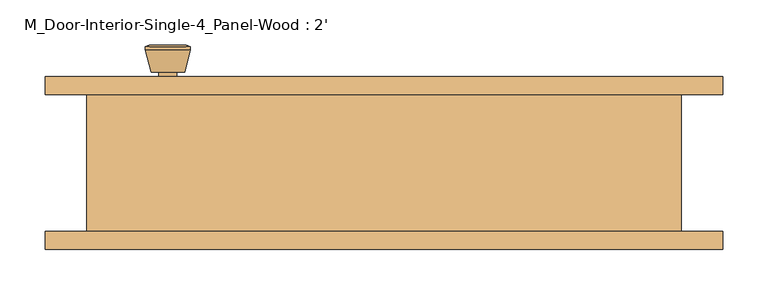
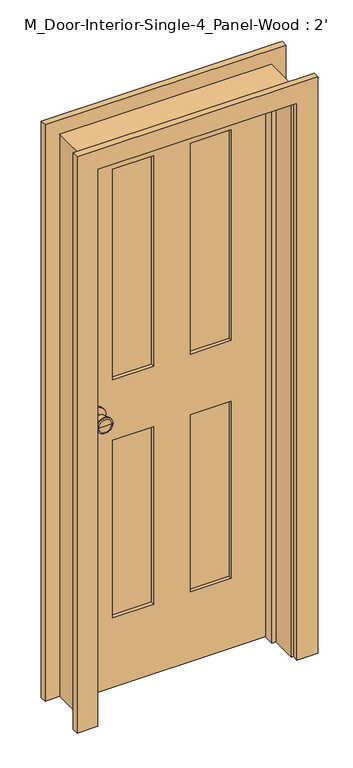
"""IFC4 building model written with IfcOpenShell, lengths in millimetres: door geometry, M_Door-Interior-Single-4_Panel-Wood : 2'."""

from ifc_helpers import new_model, si_unit, point, frame, frame_2d, origin, place, context, project, spatial, polyline, circle_curve, trimmed, segment, composite_curve, outline, extrude, faceted_brep, source, transform, mapped, element, save
from ifc_brep_helpers import plane_surface, cylinder_surface, revolved_surface, advanced_brep


def m_door_interior_single_4_panel_wood_2_0346d007(model_context):
    return source(origin(), model_context, "Body", "SolidModel", [
        advanced_brep(
        [(-239.8, 32.025, 914.4), (-229.8, 32.025, 914.4), (-249.8, 32.025, 914.4), (-219.3241324, -16.975, 914.4), (-239.8, -16.975, 914.4), (-260.2758676, -16.975, 914.4), (-214.8, -15.1471319, 914.4), (-264.8, -15.1471319, 914.4), (-214.8, -11.6834537, 914.4), (-264.8, -11.6834537, 914.4), (-221.163764, 13.025, 914.4), (-258.436236, 13.025, 914.4), (-229.8, 13.025, 914.4), (-249.8, 13.025, 914.4)],
        [
            (0, 1),
            (1, 2, circle_curve(frame((-239.8, 32.025, 914.4), z_axis=(0.0, 1.0, 0.0), x_axis=(-1.0, 0.0, 0.0)), 10.0)),
            (2, 0),
            (2, 1, circle_curve(frame((-239.8, 32.025, 914.4), z_axis=(0.0, 1.0, 0.0), x_axis=(-1.0, 0.0, 0.0)), 10.0)),
            (3, 4),
            (4, 5),
            (5, 3, circle_curve(frame((-239.8, -16.975, 914.4), z_axis=(0.0, -1.0, 0.0), x_axis=(-1.0, 0.0, 0.0)), 20.4758676)),
            (3, 5, circle_curve(frame((-239.8, -16.975, 914.4), z_axis=(0.0, -1.0, 0.0), x_axis=(-1.0, 0.0, 0.0)), 20.4758676)),
            (6, 3),
            (5, 7),
            (7, 6, circle_curve(frame((-239.8, -15.1471319, 914.4), z_axis=(0.0, -1.0, 0.0), x_axis=(-1.0, 0.0, 0.0)), 25.0)),
            (6, 7, circle_curve(frame((-239.8, -15.1471319, 914.4), z_axis=(0.0, -1.0, 0.0), x_axis=(-1.0, 0.0, 0.0)), 25.0)),
            (8, 6),
            (7, 9),
            (9, 8, circle_curve(frame((-239.8, -11.6834537, 914.4), z_axis=(0.0, -1.0, 0.0), x_axis=(-1.0, 0.0, 0.0)), 25.0)),
            (8, 9, circle_curve(frame((-239.8, -11.6834537, 914.4), z_axis=(0.0, -1.0, 0.0), x_axis=(-1.0, 0.0, 0.0)), 25.0)),
            (10, 8),
            (9, 11),
            (11, 10, circle_curve(frame((-239.8, 13.025, 914.4), z_axis=(0.0, -1.0, 0.0), x_axis=(-1.0, 0.0, 0.0)), 18.636236)),
            (10, 11, circle_curve(frame((-239.8, 13.025, 914.4), z_axis=(0.0, -1.0, 0.0), x_axis=(-1.0, 0.0, 0.0)), 18.636236)),
            (12, 10),
            (11, 13),
            (13, 12, circle_curve(frame((-239.8, 13.025, 914.4), z_axis=(0.0, -1.0, 0.0), x_axis=(-1.0, 0.0, 0.0)), 10.0)),
            (12, 13, circle_curve(frame((-239.8, 13.025, 914.4), z_axis=(0.0, -1.0, 0.0), x_axis=(-1.0, 0.0, 0.0)), 10.0)),
            (1, 12),
            (13, 2),
        ],
        [
            plane_surface(frame((-239.8, 32.025, 914.4), z_axis=(0.0, 1.0, 0.0), x_axis=(-1.0, 0.0, 0.0))),
            plane_surface(frame((-239.8, -16.975, 914.4), z_axis=(0.0, -1.0, 0.0), x_axis=(-1.0, 0.0, 0.0))),
            revolved_surface(polyline([(-260.2758676, -16.975, 914.4), (-264.8, -15.1471319, 914.4)]), (-239.8, 32.025, 914.4), (0.0, 1.0, 0.0)),
            cylinder_surface(frame((-239.8, 32.025, 914.4), z_axis=(0.0, 1.0, 0.0), x_axis=(-1.0, 0.0, 0.0)), 25.0),
            revolved_surface(polyline([(-264.8, -11.6834537, 914.4), (-258.436236, 13.025, 914.4)]), (-239.8, 32.025, 914.4), (0.0, 1.0, 0.0)),
            plane_surface(frame((-239.8, 13.025, 914.4), z_axis=(0.0, 1.0, 0.0), x_axis=(-1.0, 0.0, 0.0))),
            cylinder_surface(frame((-239.8, 32.025, 914.4), z_axis=(0.0, 1.0, 0.0), x_axis=(-1.0, 0.0, 0.0)), 10.0),
        ],
        [
            (0, [[1, 2, 3]]),
            (0, [[-3, 4, -1]]),
            (1, [[5, 6, 7]]),
            (1, [[-6, -5, 8]]),
            (2, [[9, -7, 10, 11]]),
            (2, [[-10, -8, -9, 12]]),
            (3, [[13, -11, 14, 15]]),
            (3, [[-14, -12, -13, 16]]),
            (4, [[17, -15, 18, 19]]),
            (4, [[-18, -16, -17, 20]]),
            (5, [[21, -19, 22, 23]]),
            (5, [[-22, -20, -21, 24]]),
            (6, [[25, -23, 26, -2]]),
            (6, [[-26, -24, -25, -4]]),
        ],
    ),
        extrude(outline(composite_curve([segment(trimmed(circle_curve(frame_2d((914.4, -239.8)), 30.0), [point((914.4, -269.8))], [point((914.4, -209.8))], False, "CARTESIAN"), True, "CONTINUOUS"), segment(trimmed(circle_curve(frame_2d((914.4, -239.8)), 30.0), [point((914.4, -209.8))], [point((914.4, -269.8))], False, "CARTESIAN"), True, "CONTINUOUS")], self_intersect=False)), frame((0.0, 32.025, 0.0), z_axis=(0.0, 1.0, 0.0), x_axis=(0.0, 0.0, 1.0)), (0.0, 0.0, 1.0), 6.0),
        advanced_brep(
        [(-239.8, 79.025, 914.4), (-249.8, 79.025, 914.4), (-229.8, 79.025, 914.4), (-219.3241324, 128.025, 914.4), (-260.2758676, 128.025, 914.4), (-239.8, 128.025, 914.4), (-214.8, 126.1971319, 914.4), (-264.8, 126.1971319, 914.4), (-214.8, 122.7334537, 914.4), (-264.8, 122.7334537, 914.4), (-221.163764, 98.025, 914.4), (-258.436236, 98.025, 914.4), (-229.8, 98.025, 914.4), (-249.8, 98.025, 914.4)],
        [
            (0, 1),
            (1, 2, circle_curve(frame((-239.8, 79.025, 914.4), z_axis=(0.0, -1.0, 0.0), x_axis=(-1.0, 0.0, 0.0)), 10.0)),
            (2, 0),
            (2, 1, circle_curve(frame((-239.8, 79.025, 914.4), z_axis=(0.0, -1.0, 0.0), x_axis=(-1.0, 0.0, 0.0)), 10.0)),
            (3, 4, circle_curve(frame((-239.8, 128.025, 914.4), z_axis=(0.0, 1.0, 0.0), x_axis=(-1.0, 0.0, 0.0)), 20.4758676)),
            (4, 5),
            (5, 3),
            (4, 3, circle_curve(frame((-239.8, 128.025, 914.4), z_axis=(0.0, 1.0, 0.0), x_axis=(-1.0, 0.0, 0.0)), 20.4758676)),
            (6, 7, circle_curve(frame((-239.8, 126.1971319, 914.4), z_axis=(0.0, 1.0, 0.0), x_axis=(-1.0, 0.0, 0.0)), 25.0)),
            (7, 4),
            (3, 6),
            (7, 6, circle_curve(frame((-239.8, 126.1971319, 914.4), z_axis=(0.0, 1.0, 0.0), x_axis=(-1.0, 0.0, 0.0)), 25.0)),
            (8, 9, circle_curve(frame((-239.8, 122.7334537, 914.4), z_axis=(0.0, 1.0, 0.0), x_axis=(-1.0, 0.0, 0.0)), 25.0)),
            (9, 7),
            (6, 8),
            (9, 8, circle_curve(frame((-239.8, 122.7334537, 914.4), z_axis=(0.0, 1.0, 0.0), x_axis=(-1.0, 0.0, 0.0)), 25.0)),
            (10, 11, circle_curve(frame((-239.8, 98.025, 914.4), z_axis=(0.0, 1.0, 0.0), x_axis=(-1.0, 0.0, 0.0)), 18.636236)),
            (11, 9),
            (8, 10),
            (11, 10, circle_curve(frame((-239.8, 98.025, 914.4), z_axis=(0.0, 1.0, 0.0), x_axis=(-1.0, 0.0, 0.0)), 18.636236)),
            (12, 13, circle_curve(frame((-239.8, 98.025, 914.4), z_axis=(0.0, 1.0, 0.0), x_axis=(-1.0, 0.0, 0.0)), 10.0)),
            (13, 11),
            (10, 12),
            (13, 12, circle_curve(frame((-239.8, 98.025, 914.4), z_axis=(0.0, 1.0, 0.0), x_axis=(-1.0, 0.0, 0.0)), 10.0)),
            (1, 13),
            (12, 2),
        ],
        [
            plane_surface(frame((-239.8, 79.025, 914.4), z_axis=(0.0, -1.0, 0.0), x_axis=(-1.0, 0.0, 0.0))),
            plane_surface(frame((-239.8, 128.025, 914.4), z_axis=(0.0, 1.0, 0.0), x_axis=(-1.0, 0.0, 0.0))),
            revolved_surface(polyline([(-260.2758676, 128.025, 914.4), (-264.8, 126.1971319, 914.4)]), (-239.8, 79.025, 914.4), (0.0, -1.0, 0.0)),
            cylinder_surface(frame((-239.8, 79.025, 914.4), z_axis=(0.0, -1.0, 0.0), x_axis=(-1.0, 0.0, 0.0)), 25.0),
            revolved_surface(polyline([(-264.8, 122.7334537, 914.4), (-258.436236, 98.025, 914.4)]), (-239.8, 79.025, 914.4), (0.0, -1.0, 0.0)),
            plane_surface(frame((-239.8, 98.025, 914.4), z_axis=(0.0, -1.0, 0.0), x_axis=(-1.0, 0.0, 0.0))),
            cylinder_surface(frame((-239.8, 79.025, 914.4), z_axis=(0.0, -1.0, 0.0), x_axis=(-1.0, 0.0, 0.0)), 10.0),
        ],
        [
            (0, [[1, 2, 3]]),
            (0, [[-3, 4, -1]]),
            (1, [[5, 6, 7]]),
            (1, [[8, -7, -6]]),
            (2, [[9, 10, -5, 11]]),
            (2, [[12, -11, -8, -10]]),
            (3, [[13, 14, -9, 15]]),
            (3, [[16, -15, -12, -14]]),
            (4, [[17, 18, -13, 19]]),
            (4, [[20, -19, -16, -18]]),
            (5, [[21, 22, -17, 23]]),
            (5, [[24, -23, -20, -22]]),
            (6, [[-2, 25, -21, 26]]),
            (6, [[-4, -26, -24, -25]]),
        ],
    ),
        extrude(outline(composite_curve([segment(trimmed(circle_curve(frame_2d((914.4, -239.8)), 30.0), [point((914.4, -269.8))], [point((914.4, -209.8))], False, "CARTESIAN"), True, "CONTINUOUS"), segment(trimmed(circle_curve(frame_2d((914.4, -239.8)), 30.0), [point((914.4, -209.8))], [point((914.4, -269.8))], False, "CARTESIAN"), True, "CONTINUOUS")], self_intersect=False)), frame((0.0, 73.025, 0.0), z_axis=(0.0, 1.0, 0.0), x_axis=(0.0, 0.0, 1.0)), (0.0, 0.0, 1.0), 6.0),
        faceted_brep([(329.8, 73.025, 0.0), (329.8, -79.375, 0.0), (304.8, -79.375, 0.0), (304.8, 3.1, 0.0), (292.1, 3.1, 0.0), (292.1, 38.025, 0.0), (304.8, 38.025, 0.0), (304.8, 73.025, 0.0), (329.8, 73.025, 1853.8), (329.8, -79.375, 1853.8), (-329.8, -79.375, 1853.8), (-329.8, -79.375, 0.0), (-304.8, -79.375, 0.0), (-304.8, -79.375, 1828.8), (304.8, -79.375, 1828.8), (304.8, 3.1, 1828.8), (-304.8, 3.1, 1828.8), (-304.8, 3.1, 0.0), (-292.1, 3.1, 0.0), (-292.1, 3.1, 1816.1), (292.1, 3.1, 1816.1), (292.1, 38.025, 1816.1), (-292.1, 38.025, 1816.1), (-292.1, 38.025, 0.0), (-304.8, 38.025, 0.0), (-304.8, 38.025, 1828.8), (304.8, 38.025, 1828.8), (304.8, 73.025, 1828.8), (-304.8, 73.025, 1828.8), (-304.8, 73.025, 0.0), (-329.8, 73.025, 0.0), (-329.8, 73.025, 1853.8)], [[[0, 1, 2, 3, 4, 5, 6, 7]], [[1, 0, 8, 9]], [[2, 1, 9, 10, 11, 12, 13, 14]], [[3, 2, 14, 15]], [[4, 3, 15, 16, 17, 18, 19, 20]], [[5, 4, 20, 21]], [[6, 5, 21, 22, 23, 24, 25, 26]], [[7, 6, 26, 27]], [[0, 7, 27, 28, 29, 30, 31, 8]], [[9, 8, 31, 10]], [[15, 14, 13, 16]], [[21, 20, 19, 22]], [[27, 26, 25, 28]], [[30, 29, 24, 23, 18, 17, 12, 11]], [[10, 31, 30, 11]], [[16, 13, 12, 17]], [[22, 19, 18, 23]], [[28, 25, 24, 29]]]),
        extrude(outline(polyline([(1828.8, -304.8), (0.0, -304.8), (0.0, 304.8), (1828.8, 304.8), (1828.8, -304.8)]), holes=[polyline([(1708.8, 57.5), (1708.8, 184.8), (1014.4, 184.8), (1014.4, 57.5), (1708.8, 57.5)]), polyline([(1014.4, -57.5), (1014.4, -184.8), (1708.8, -184.8), (1708.8, -57.5), (1014.4, -57.5)]), polyline([(814.4, 57.5), (814.4, 184.8), (230.0, 184.8), (230.0, 57.5), (814.4, 57.5)]), polyline([(230.0, -57.5), (230.0, -184.8), (814.4, -184.8), (814.4, -57.5), (230.0, -57.5)])]), frame((0.0, 38.025, 0.0), z_axis=(0.0, 1.0, 0.0), x_axis=(0.0, 0.0, 1.0)), (0.0, 0.0, 1.0), 35.0),
        extrude(outline(polyline([(184.8, 49.6916667), (57.5, 49.6916667), (57.5, 61.3583333), (184.8, 61.3583333), (184.8, 49.6916667)])), frame((0.0, 0.0, 1014.4), z_axis=(0.0, 0.0, 1.0), x_axis=(1.0, 0.0, 0.0)), (0.0, 0.0, 1.0), 694.4),
        extrude(outline(polyline([(-57.5, 49.6916667), (-184.8, 49.6916667), (-184.8, 61.3583333), (-57.5, 61.3583333), (-57.5, 49.6916667)])), frame((0.0, 0.0, 1014.4), z_axis=(0.0, 0.0, 1.0), x_axis=(1.0, 0.0, 0.0)), (0.0, 0.0, 1.0), 694.4),
        extrude(outline(polyline([(184.8, 49.6916667), (57.5, 49.6916667), (57.5, 61.3583333), (184.8, 61.3583333), (184.8, 49.6916667)])), frame((0.0, 0.0, 230.0), z_axis=(0.0, 0.0, 1.0), x_axis=(1.0, 0.0, 0.0)), (0.0, 0.0, 1.0), 584.4),
        extrude(outline(polyline([(-57.5, 49.6916667), (-184.8, 49.6916667), (-184.8, 61.3583333), (-57.5, 61.3583333), (-57.5, 49.6916667)])), frame((0.0, 0.0, 230.0), z_axis=(0.0, 0.0, 1.0), x_axis=(1.0, 0.0, 0.0)), (0.0, 0.0, 1.0), 584.4),
        extrude(outline(polyline([(0.0, 311.15), (0.0, 376.15), (1900.15, 376.15), (1900.15, -376.15), (0.0, -376.15), (0.0, -311.15), (1835.15, -311.15), (1835.15, 311.15), (0.0, 311.15)])), frame((0.0, 73.025, 0.0), z_axis=(0.0, 1.0, 0.0), x_axis=(0.0, 0.0, 1.0)), (0.0, 0.0, 1.0), 20.0),
        extrude(outline(polyline([(0.0, 311.15), (0.0, 376.15), (1900.15, 376.15), (1900.15, -376.15), (0.0, -376.15), (0.0, -311.15), (1835.15, -311.15), (1835.15, 311.15), (0.0, 311.15)])), frame((0.0, -99.375, 0.0), z_axis=(0.0, 1.0, 0.0), x_axis=(0.0, 0.0, 1.0)), (0.0, 0.0, 1.0), 20.0),
    ])


if __name__ == "__main__":
    model = new_model("IFC4")
    model_context = context("Model", 3, world=origin())
    ifc_project = project(units=[si_unit("LENGTHUNIT", "METRE", prefix="MILLI")], contexts=[model_context])
    site = spatial("IfcSite", under=ifc_project)
    building = spatial("IfcBuilding", under=site)
    placement = place(None, origin())
    m_door_interior_single_4_panel_wood_2_shape = m_door_interior_single_4_panel_wood_2_0346d007(model_context)
    element("IfcDoor", 1, ObjectType="M_Door-Interior-Single-4_Panel-Wood : 2'", at=placement, inside=building, context=model_context, shape_type="MappedRepresentation", body=[
        mapped(m_door_interior_single_4_panel_wood_2_shape, transform((0.0, 0.0, 0.0), x_axis=(1.0, 0.0, 0.0), y_axis=(0.0, 1.0, 0.0), z_axis=(0.0, 0.0, 1.0))),
    ])
    save(model, "model.ifc")

# Revit data of these elements
# Type "M_Door-Interior-Single-4_Panel-Wood : 2'"
#   Type Mark = "13"
#   Assembly Code = "C1020300"
#   Analytic Construction = "Wooden"
#   Top Rail = 0' - 4.72441"
#   Thickness = 0' - 1.37795"
#   Thermal Resistance (R) = 2.5876 (h·ft²·°F)/BTU
#   Swing Angle [instance default] = 90.00°
#   Stiles = 0' - 4.72441"
#   Rough Width = 2' - 1.9685"
#   Rough Height = 6' - 0.98425"
#   Mullion = 0' - 4.52756"
#   Lock Rail = 0' - 7.87402"
#   Height = 6' - 0"
#   Width = 2' - 0"
#   Heat Transfer Coefficient (U) = 0.3865 BTU/(h·ft²·°F)
#   Bottom Rail = 0' - 9.05512"
#   Trim Material = Cherry
#   Panel Material = Cherry
#   Frame Material = Cherry
#   Door Handle Material = Aluminum
#   Visual Light Transmittance = 0
#   Solar Heat Gain Coefficient = 0
#   Wall Closure = (empty or 0)
#   Function = (empty or 0)
# Element 1 (IfcDoor, "M_Door-Interior-Single-4_Panel-Wood : 2'")
#   Materials on its faces: "Cherry", "Aluminum"
# Materials
#   "Cherry": class "Wood", colour RGB 226 177 128, transparency 0, Description = "Prunus Serotina", Cost = 0
#   "Aluminum": class "Metal", colour RGB 247 247 247, transparency 0, Description = "Aluminum 6061", Cost = 0
